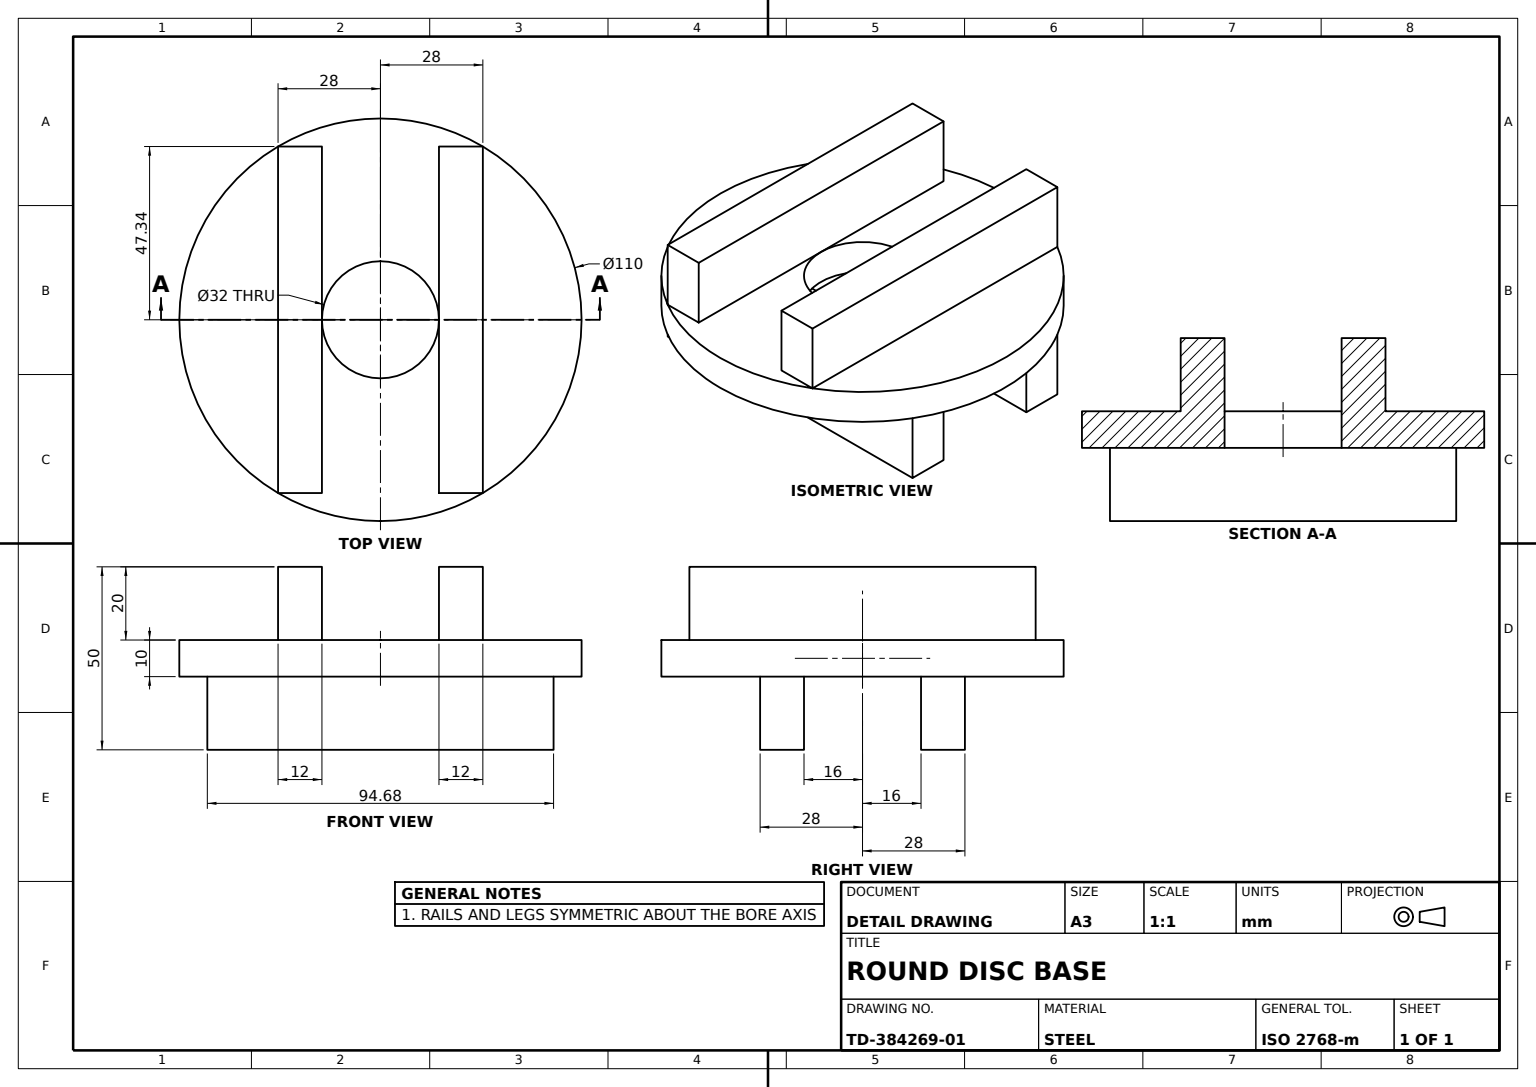
from build123d import *

# Parameters (mm, degrees)
BASE_DISC_SKETCH_R          = 55
BASE_DISC_SKETCH_R_2        = 16
BASE_DISC_110_BORE_32_DEPTH = 10
TOP_RAILS_SKETCH_W          = 12
TOP_RAILS_SKETCH_H          = 94.678403028
TOP_RAILS_DEPTH             = 20
BOTTOM_LEGS_SKETCH_W        = 94.678403028
BOTTOM_LEGS_SKETCH_H        = 12
BOTTOM_LEGS_DEPTH           = 20


with BuildPart() as part:
    # Base Disc Sketch → Base Disc Ø110 Bore Ø32 (new body)
    with BuildSketch(Plane(origin=(0, 0, 0), x_dir=(1, 0, 0), z_dir=(0, 1, 0))):
        with Locations(Location((0, 0, 0), (0, 0, 270))):
            Circle(BASE_DISC_SKETCH_R)
        with Locations(Location((0, 0, 0), (0, 0, 270))):
            Circle(BASE_DISC_SKETCH_R_2, mode=Mode.SUBTRACT)
    extrude(amount=BASE_DISC_110_BORE_32_DEPTH)

    # Top Rails Sketch → Top Rails (add)
    with BuildSketch(Plane(origin=(0, 10, 0), x_dir=(1, 0, 0), z_dir=(0, 1, 0))):
        with Locations((22, 0)):
            Rectangle(TOP_RAILS_SKETCH_W, TOP_RAILS_SKETCH_H)
        with Locations((-22, 0)):
            Rectangle(TOP_RAILS_SKETCH_W, TOP_RAILS_SKETCH_H)
    extrude(amount=TOP_RAILS_DEPTH)

    # Bottom Legs Sketch → Bottom Legs (add)
    with BuildSketch(Plane.XZ):
        with Locations((0, 22)):
            Rectangle(BOTTOM_LEGS_SKETCH_W, BOTTOM_LEGS_SKETCH_H)
        with Locations((0, -22)):
            Rectangle(BOTTOM_LEGS_SKETCH_W, BOTTOM_LEGS_SKETCH_H)
    extrude(amount=BOTTOM_LEGS_DEPTH)


solid = part.part
